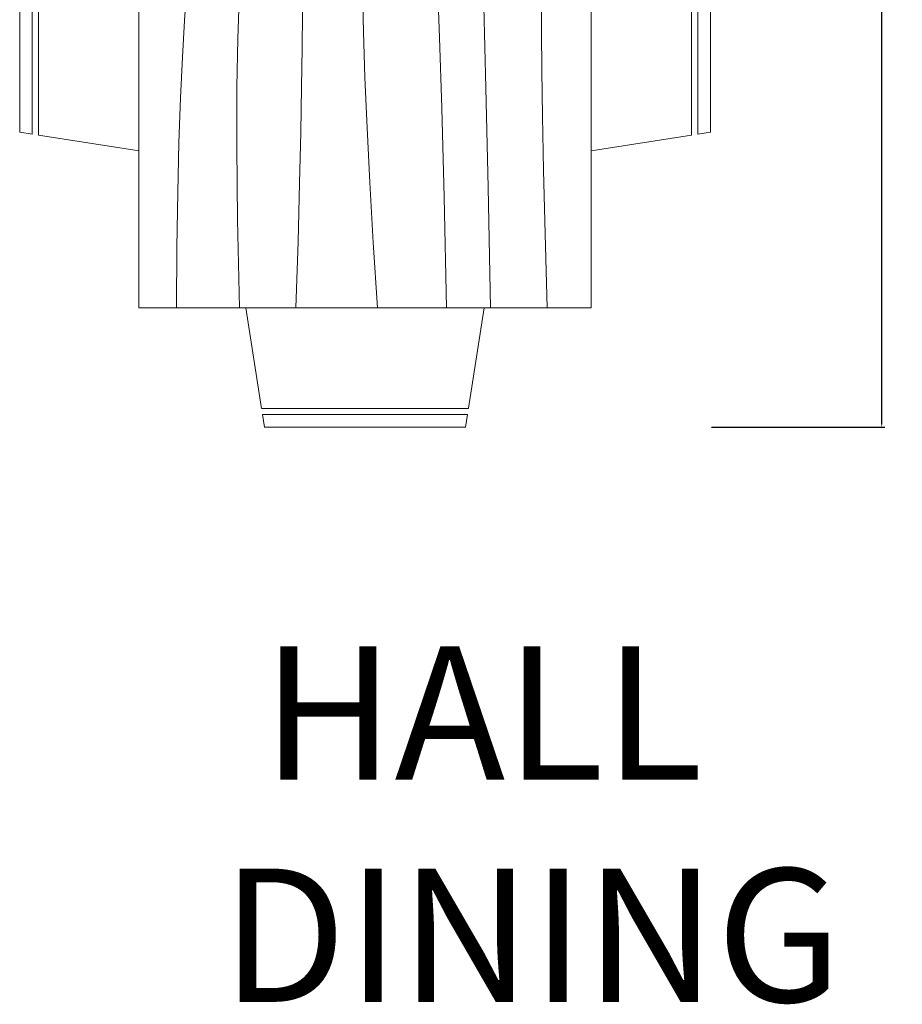
# Model space of a CAD drawing. Units: inches. Extents: x -301 to 715, y -607 to 364.
# Tile 105 of 141: x -41 to 12, y 88 to 147. Entities that reach past the tile are written whole.
import ezdxf

# ---------------------------------------------------------------- set-up
doc = ezdxf.new("R2010")
doc.units = ezdxf.units.IN
doc.header["$MEASUREMENT"] = 0
for name, color, linetype, lineweight in [('A-ANNO-DIMS', 2, 'Continuous', 18), ('A-AREA-IDEN', 220, 'Continuous', 25), ('A-FURN', 8, 'Continuous', 18)]:
    doc.layers.add(name, color=color, linetype=linetype, lineweight=lineweight)
doc.styles.get("Standard").update_dxf_attribs({"font": 'arial.ttf'})
doc.dimstyles.get("Standard").update_dxf_attribs({"dimtxt": 0.18, "dimasz": 0.18, "dimexe": 0.18, "dimexo": 0.0625, "dimgap": 0.09, "dimtad": 0, "dimtih": 1, "dimtoh": 1, "dimdec": 1, "dimzin": 0, "dimdsep": 46, "dimlunit": 4, "dimtxsty": 'Standard', "dimcen": 0.09, "dimclrd": 3, "dimclre": 4, "dimclrt": 6, "dimadec": 0, "dimazin": 0, "dimtfac": 1, "dimtdec": 1, "dimtofl": 0, "dimtmove": 0, "dimatfit": 3, "dimfxl": 1, "dimtfill": 2, "dimtfillclr": 51, "dimtolj": 1, "dimtzin": 0, "dimarcsym": 0})

# ---------------------------------------------------------------- blocks, each defined once
blk = doc.blocks.new('Dining Set - 36 x 72 in.')
for p, q in [((-22, 27.5), (-22.1562, 26.50042)), ((-22, 27.5), (-6, 27.5)), ((-5.8437, 26.49966), (-6, 27.5)), ((6, 27.5), (5.8438, 26.50042)), ((6, 27.5), (22, 27.5)), ((22.1563, 26.49966), (22, 27.5)), ((-22.2343, 26.00059), (-23.4847, 17.99762)), ((-22.2304, 26), (-5.7608, 26)), ((-5.8416, 26.5), (-22.1534, 26.5)), ((-4.5152, 17.99762), (-5.7655, 25.99926)), ((5.7657, 26.00059), (4.5153, 17.99762)), ((5.7696, 26), (22.2392, 26)), ((22.1584, 26.5), (5.8466, 26.5)), ((23.4848, 17.99762), (22.2345, 25.99926)), ((36, 18), (-36, 18)), ((-36, 18), (-36, -18)), ((36, -18), (36, 18)), ((-44.0006, 8.23428), (-35.9976, 9.48474)), ((44.0006, 8.23428), (35.9976, 9.48474)), ((-45.5, 8), (-44.5004, 8.15617)), ((-45.5, 8), (-45.5, -8)), ((-44.5, -8.15843), (-44.5, 8.15338)), ((-44, 8.23041), (-44, -8.23915)), ((44, 8.23041), (44, -8.23915)), ((44.5, -8.15843), (44.5, 8.15338)), ((45.5, 8), (44.5005, 8.15617)), ((45.5, 8), (45.5, -8)), ((-44.4997, -8.15631), (-45.5, -8)), ((-35.9976, -9.48476), (-43.9993, -8.2345)), ((35.9976, -9.48476), (43.9993, -8.2345)), ((44.4997, -8.15631), (45.5, -8)), ((-36, -18), (36, -18)), ((-22.2343, -26.0006), (-23.4847, -17.99762)), ((-4.5152, -17.99762), (-5.7655, -25.99928)), ((5.7657, -26.0006), (4.5153, -17.99762)), ((23.4848, -17.99762), (22.2345, -25.99928)), ((-22.2304, -26), (-5.7608, -26)), ((-22, -27.5), (-22.1562, -26.50044)), ((-5.8416, -26.5), (-22.1534, -26.5)), ((-5.8437, -26.49967), (-6, -27.5)), ((5.7696, -26), (22.2392, -26)), ((6, -27.5), (5.8438, -26.50044)), ((22.1584, -26.5), (5.8466, -26.5)), ((22.1563, -26.49967), (22, -27.5)), ((-22, -27.5), (-6, -27.5)), ((6, -27.5), (22, -27.5))]:
    blk.add_line(p, q)
for points in [[(-36, 15), (-31.1772, 14.97754), (-26.8079, 14.91406), (-22.8538, 14.81543), (-19.276, 14.6875), (-16.0362, 14.53613), (-13.0957, 14.36718), (-10.4159, 14.18652), (-7.9583, 14), (-5.6904, 13.81315), (-3.6035, 13.63021), (-1.6954, 13.45508), (0.0365, 13.29166), (1.5945, 13.14388), (2.9811, 13.01562), (4.1988, 12.9108), (5.25, 12.83333), (6.1393, 12.78613), (6.8802, 12.76823), (7.4883, 12.77767), (7.9792, 12.8125), (8.3685, 12.87077), (8.6719, 12.95052), (8.9049, 13.0498), (9.0833, 13.16666), (9.2205, 13.29899), (9.3216, 13.44401), (9.3895, 13.59879), (9.4271, 13.76041), (9.4373, 13.92594), (9.4232, 14.09245), (9.3875, 14.257), (9.3333, 14.41666), (9.2638, 14.56917), (9.1836, 14.71484), (9.0975, 14.85465), (9.0104, 14.98958), (8.9272, 15.1206), (8.8529, 15.2487), (8.7922, 15.37483), (8.75, 15.5), (8.7305, 15.62467), (8.7344, 15.74739), (8.7617, 15.86621), (8.8125, 15.97916), (8.8867, 16.08431), (8.9844, 16.17968), (9.1055, 16.26334), (9.25, 16.33333), (9.4189, 16.38802), (9.6172, 16.42708), (9.8506, 16.45052), (10.125, 16.45833), (10.4463, 16.45052), (10.8203, 16.42708), (11.2529, 16.38802), (11.75, 16.33333), (12.3184, 16.26318), (12.9694, 16.17838), (13.7151, 16.07991), (14.5677, 15.96875), (15.5395, 15.84586), (16.6426, 15.71224), (17.8893, 15.56884), (19.2917, 15.41666), (20.859, 15.25667), (22.5879, 15.08984), (24.4721, 14.91715), (26.5052, 14.73958), (28.6809, 14.5581), (30.9929, 14.3737), (33.4347, 14.18733), (36, 14)], [(-36, 10), (-28.9766, 10.14274), (-23.1725, 10.20442), (-18.4241, 10.19775), (-14.5677, 10.13541), (-11.4399, 10.03011), (-8.877, 9.89453), (-6.7154, 9.74137), (-4.7917, 9.58333), (-2.9698, 9.43082), (-1.2246, 9.28515), (0.4415, 9.14534), (2.026, 9.01041), (3.5266, 8.87939), (4.9408, 8.7513), (6.266, 8.62516), (7.5, 8.5), (8.6411, 8.37549), (9.6914, 8.2539), (10.6538, 8.13818), (11.5312, 8.03125), (12.3267, 7.93603), (13.043, 7.85547), (13.6831, 7.79248), (14.25, 7.75), (14.7471, 7.7303), (15.1797, 7.73307), (15.5537, 7.75732), (15.875, 7.80208), (16.1494, 7.86637), (16.3828, 7.94922), (16.5811, 8.04964), (16.75, 8.16666), (16.8944, 8.29915), (17.0143, 8.44531), (17.1089, 8.60319), (17.1771, 8.77083), (17.218, 8.94629), (17.2305, 9.1276), (17.2137, 9.31282), (17.1667, 9.5), (17.0895, 9.6875), (16.987, 9.875), (16.8649, 10.0625), (16.7292, 10.25), (16.5856, 10.4375), (16.4401, 10.625), (16.2985, 10.8125), (16.1667, 11), (16.05, 11.18733), (15.9518, 11.3737), (15.8752, 11.5581), (15.8229, 11.73958), (15.798, 11.91715), (15.8034, 12.08984), (15.842, 12.25667), (15.9167, 12.41666), (16.0295, 12.56836), (16.1784, 12.70833), (16.3605, 12.83268), (16.5729, 12.9375), (16.8127, 13.01888), (17.0768, 13.07291), (17.3625, 13.0957), (17.6667, 13.08333), (17.9894, 13.03312), (18.3418, 12.94726), (18.7382, 12.82918), (19.1927, 12.68229), (19.7195, 12.51001), (20.3327, 12.31575), (21.0465, 12.10294), (21.875, 11.875), (22.8357, 11.63354), (23.959, 11.37304), (25.2786, 11.08618), (26.8282, 10.76562), (28.6414, 10.40405), (30.752, 9.99414), (33.1936, 9.52856), (36, 9)], [(-36, 5.5), (-30.7157, 5.3348), (-26.069, 5.20963), (-21.9946, 5.11767), (-18.4271, 5.05208), (-15.3009, 5.00602), (-12.5508, 4.97265), (-10.1112, 4.94515), (-7.9167, 4.91666), (-5.909, 4.88167), (-4.0586, 4.83984), (-2.3429, 4.79215), (-0.7396, 4.73958), (0.7739, 4.6831), (2.22, 4.6237), (3.6213, 4.56233), (5, 4.5), (6.373, 4.43782), (7.7344, 4.3776), (9.0723, 4.32129), (10.375, 4.27083), (11.6309, 4.22819), (12.8281, 4.19531), (13.9551, 4.17415), (15, 4.16666), (15.954, 4.17448), (16.819, 4.19791), (17.6001, 4.23698), (18.3021, 4.29166), (18.9299, 4.36198), (19.4883, 4.44791), (19.9823, 4.54948), (20.4167, 4.66666), (20.7969, 4.79899), (21.1302, 4.94401), (21.4245, 5.09879), (21.6875, 5.26041), (21.9271, 5.42594), (22.1511, 5.59245), (22.3672, 5.757), (22.5834, 5.91666), (22.8065, 6.06868), (23.0404, 6.21093), (23.2879, 6.34147), (23.5521, 6.45833), (23.8358, 6.55957), (24.142, 6.64323), (24.4735, 6.70735), (24.8334, 6.75), (25.2235, 6.76969), (25.642, 6.76692), (26.0858, 6.74267), (26.5521, 6.69791), (27.0379, 6.63362), (27.5404, 6.55078), (28.0565, 6.45036), (28.5834, 6.33333), (29.1242, 6.19987), (29.7071, 6.04687), (30.3661, 5.87044), (31.1354, 5.66666), (32.0493, 5.43164), (33.142, 5.16146), (34.4475, 4.85221), (36, 4.5)], [(-36, -1), (-30.7915, -0.6591), (-26.0195, -0.38216), (-21.6519, -0.16284), (-17.6563, 0.00521), (-14.0005, 0.12833), (-10.6523, 0.21289), (-7.5796, 0.26522), (-4.75, 0.29166), (-2.134, 0.29793), (0.2878, 0.28711), (2.5317, 0.26163), (4.6146, 0.22396), (6.5529, 0.17651), (8.3633, 0.12174), (10.0623, 0.06209), (11.6667, 0), (13.1899, -0.06201), (14.6341, -0.1211), (15.9982, -0.17432), (17.2813, -0.21875), (18.4823, -0.25147), (19.6003, -0.26953), (20.6343, -0.27002), (21.5834, -0.25), (22.4481, -0.20768), (23.2357, -0.14584), (23.9549, -0.06836), (24.6146, 0.02083), (25.2235, 0.11784), (25.7904, 0.21875), (26.3241, 0.31966), (26.8334, 0.41666), (27.3265, 0.50618), (27.8099, 0.58593), (28.2894, 0.65397), (28.7709, 0.70833), (29.2601, 0.74707), (29.763, 0.76823), (30.2855, 0.76985), (30.8334, 0.75), (31.4088, 0.70784), (31.9994, 0.64713), (32.589, 0.57275), (33.1615, 0.48958), (33.7008, 0.4025), (34.1908, 0.3164), (34.6153, 0.23616), (34.9584, 0.16666), (35.2099, 0.11165), (35.3848, 0.07031), (35.504, 0.04069), (35.5886, 0.02083), (35.6594, 0.00879), (35.7377, 0.0026), (35.8442, 0.00032), (36, 0)], [(-36, -6.5), (-27.1843, -6.31267), (-20.084, -6.1263), (-14.469, -5.9419), (-10.1094, -5.76042), (-6.7752, -5.58285), (-4.2363, -5.41016), (-2.2629, -5.24333), (-0.625, -5.08334), (0.8708, -4.93099), (2.2715, -4.78646), (3.5872, -4.64974), (4.8281, -4.52084), (6.0046, -4.39974), (7.127, -4.28646), (8.2053, -4.18099), (9.25, -4.08334), (10.2705, -3.99382), (11.2734, -3.91407), (12.2647, -3.84603), (13.25, -3.79167), (14.2354, -3.75293), (15.2266, -3.73177), (16.2295, -3.73015), (17.25, -3.75), (18.2912, -3.79248), (19.3451, -3.85547), (20.4009, -3.93604), (21.4479, -4.03125), (22.4754, -4.13819), (23.4727, -4.25391), (24.4289, -4.37549), (25.3334, -4.5), (26.1785, -4.62492), (26.9694, -4.74935), (27.7145, -4.87281), (28.4219, -4.99479), (29.1, -5.11483), (29.7572, -5.23242), (30.4016, -5.34709), (31.0417, -5.45834), (31.6837, -5.56437), (32.3262, -5.65821), (32.9658, -5.73153), (33.599, -5.77604), (34.2224, -5.78345), (34.8327, -5.74545), (35.4264, -5.65373), (36, -5.5)], [(-36, -10), (-26.4022, -9.81299), (-18.4675, -9.62891), (-11.9839, -9.45069), (-6.7396, -9.28125), (-2.5226, -9.12354), (0.8789, -8.98047), (3.6769, -8.85498), (6.0833, -8.75), (8.2767, -8.66765), (10.3021, -8.60677), (12.1712, -8.56543), (13.8958, -8.54167), (15.4876, -8.53353), (16.9583, -8.53907), (18.3197, -8.55632), (19.5834, -8.58334), (20.7616, -8.61841), (21.8685, -8.66081), (22.9188, -8.71004), (23.9271, -8.76563), (24.9081, -8.82707), (25.8763, -8.89388), (26.8465, -8.96558), (27.8334, -9.04167), (28.8474, -9.12118), (29.8828, -9.20117), (30.93, -9.27824), (31.9792, -9.34896), (33.0205, -9.40991), (34.0443, -9.45768), (35.0407, -9.48885), (36, -9.5)], [(-36, -14.5), (-30.0881, -14.33513), (-25.0332, -14.21224), (-20.7312, -14.12647), (-17.0781, -14.07292), (-13.97, -14.04671), (-11.3027, -14.04297), (-8.9724, -14.05681), (-6.875, -14.08334), (-4.9224, -14.11833), (-3.0905, -14.16016), (-1.3709, -14.20785), (0.2448, -14.26042), (1.7647, -14.3169), (3.1973, -14.3763), (4.5507, -14.43767), (5.8333, -14.5), (7.0554, -14.5621), (8.235, -14.62175), (9.3922, -14.67652), (10.5469, -14.72396), (11.7192, -14.76164), (12.929, -14.78711), (14.1965, -14.79794), (15.5417, -14.79167), (16.9933, -14.76424), (18.6152, -14.70508), (20.4804, -14.60197), (22.6615, -14.44271), (25.2312, -14.21509), (28.2624, -13.9069), (31.8277, -13.50594), (36, -13)]]:
    blk.add_lwpolyline(points)
blk = doc.blocks.new('*D128')
at = {"layer": 'A-ANNO-DIMS', "color": 4, "lineweight": -2, "transparency": 16777216}
for p, q in [((0.532, 191.307), (10.93, 191.307)), ((0.532, 122.765), (10.93, 122.765))]:
    blk.add_line(p, q, dxfattribs=at)
at = {"layer": 'A-ANNO-DIMS', "color": 3, "lineweight": -2, "transparency": 16777216}
for p, q in [((10.75, 191.127), (10.75, 157.219)), ((10.75, 122.945), (10.75, 156.853))]:
    blk.add_line(p, q, dxfattribs=at)
at = {"layer": 'A-ANNO-DIMS', "color": 3, "transparency": 16777216}
for points in [[(10.72, 191.127), (10.78, 191.127), (10.75, 191.307)], [(10.72, 122.945), (10.78, 122.945), (10.75, 122.765)]]:
    blk.add_solid(points, dxfattribs=at)
at = {"layer": 'Defpoints', "color": 0, "transparency": 16777216}
for p in [(0.469, 191.307), (10.75, 191.307), (0.469, 122.765)]:
    blk.add_point(p, dxfattribs=at)
at = {"layer": 'A-ANNO-DIMS', "color": 6, "transparency": 16777216, "insert": (10.75, 157.036), "char_height": 0.18, "attachment_point": 5, "bg_fill": 1, "box_fill_scale": 1.25, "bg_fill_color": 51, "bg_fill_transparency": 0}
blk.add_mtext('\\A1;DINING SET 5\'-8 1/2"', dxfattribs=at)

msp = doc.modelspace()

# ---------------------------------------------------------------- block references
at = {"layer": 'A-FURN', "xscale": 0.753207081168398, "yscale": 0.753207081168398, "zscale": 0.753207081168398, "rotation": 90}
msp.add_blockref('Dining Set - 36 x 72 in.', (-20.244, 157.036), dxfattribs=at)

# ---------------------------------------------------------------- texts
at = {"layer": 'A-AREA-IDEN', "insert": (-28.862, 109.616), "char_height": 8, "attachment_point": 1}
msp.add_mtext_dynamic_manual_height_columns(' HALL\\PDINING', width=73.06001, gutter_width=1, heights=[0], dxfattribs=at)

# ---------------------------------------------------------------- dimensions: what is measured, and where the dimension line sits
at = {"layer": 'A-ANNO-DIMS'}
dim = msp.add_linear_dim(base=(10.75, 191.307), p1=(0.469, 122.765), p2=(0.469, 191.307), angle=90, text='DINING SET <>', dimstyle='Standard', override={"dimdec": 1, "dimlfac": 1, "dimrnd": 0, "dimzin": 1, "dimdsep": 46, "dimlunit": 4, "dimfrac": 2}, dxfattribs=at)
dim.commit()
dim.dimension.update_dxf_attribs({"geometry": '*D128', "text_midpoint": (10.75, 157.036)})

doc.saveas('drawing.dxf')
